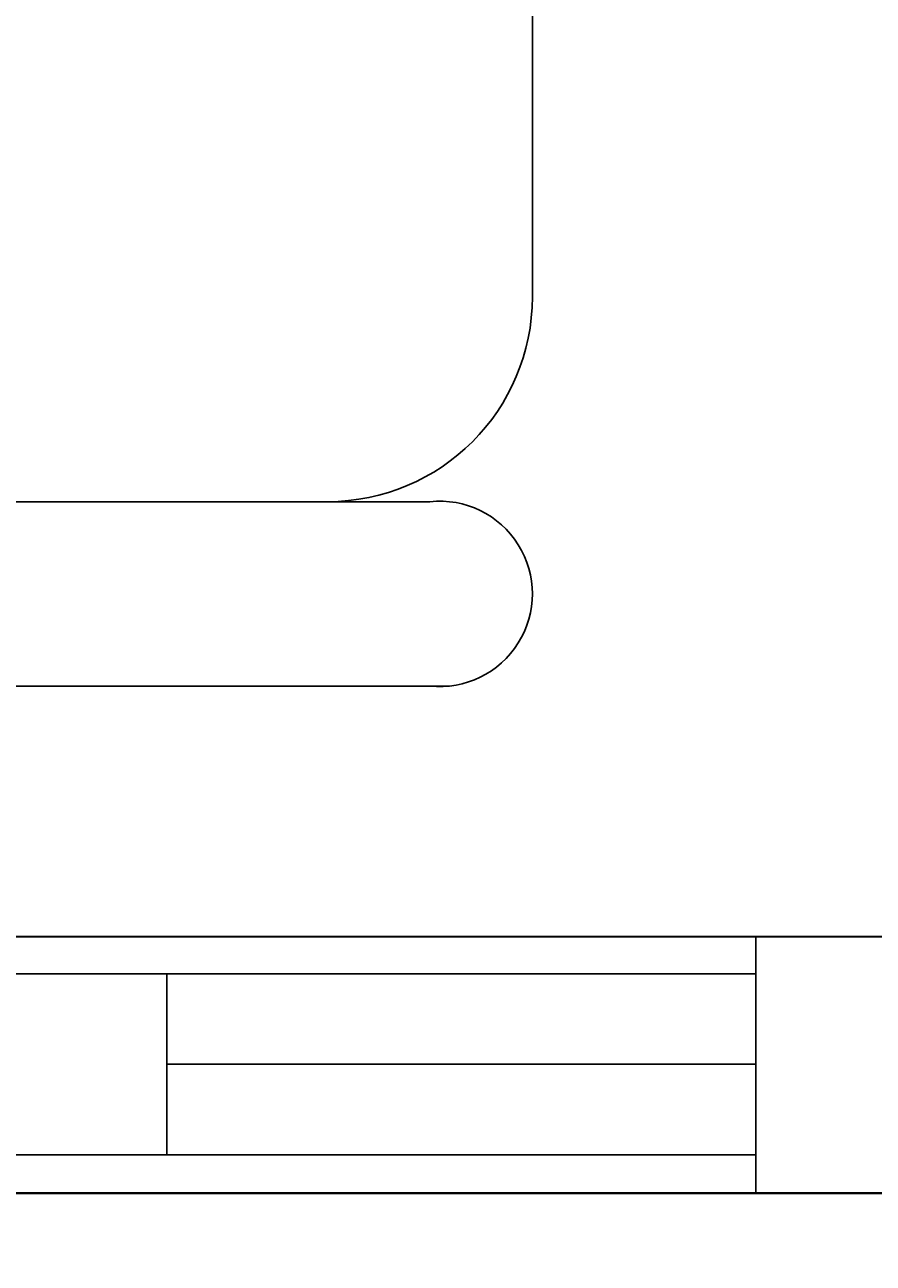
# Model space of a CAD drawing. Units: millimetres. Extents: x 19292 to 100733, y 12374 to 26974.
# Tile 4 of 24: x 28279 to 29028, y 14845 to 15938. Entities that reach past the tile are written whole.
import ezdxf

# ---------------------------------------------------------------- set-up
doc = ezdxf.new("R2010")
doc.units = ezdxf.units.MM
for name, color, linetype, lineweight in [('A-ANNO-DIMS', 2, 'Continuous', 18), ('A-FLOR-PATT', 252, 'Continuous', 13), ('A-FURN', 8, 'Continuous', 18), ('A-GLAZ', 3, 'Continuous', 25), ('A-WALL', 7, 'Continuous', 35)]:
    doc.layers.add(name, color=color, linetype=linetype, lineweight=lineweight)
doc.layers.add('FURNITURE', color=40, linetype='Continuous')
doc.layers.add('WINDOWS', color=50, linetype='Continuous')
doc.styles.get("Standard").update_dxf_attribs({"font": 'arial.ttf'})
doc.dimstyles.get("Standard").update_dxf_attribs({"dimtxt": 0.18, "dimasz": 0.18, "dimexe": 0.18, "dimexo": 0.0625, "dimgap": 0.09, "dimtad": 0, "dimtih": 1, "dimtoh": 1, "dimdec": 4, "dimzin": 0, "dimdsep": 46, "dimtxsty": 'Standard', "dimcen": 0.09, "dimadec": 0, "dimazin": 0, "dimtfac": 1, "dimtdec": 4, "dimtofl": 0, "dimtmove": 0, "dimatfit": 3, "dimfxl": 1, "dimtolj": 1, "dimtzin": 0, "dimarcsym": 0})

# ---------------------------------------------------------------- blocks, each defined once
blk = doc.blocks.new('WW')
at = {"layer": 'WINDOWS'}
for p, q in [((-5183.9, -4940.9), (-3983.9, -4940.9)), ((-4663.9, -4940.9), (-4663.9, -5100.9)), ((-4503.9, -4940.9), (-4503.9, -5100.9)), ((-4503.9, -4940.9), (-4503.9, -5100.9)), ((-5183.9, -5020.9), (-4663.9, -5020.9)), ((-4503.9, -5020.9), (-3983.9, -5020.9)), ((-5183.9, -5100.9), (-3983.9, -5100.9))]:
    blk.add_line(p, q, dxfattribs=at)
for points in [[(-5183.9, -5133.4), (-5183.9, -4908.4)], [(-3983.9, -4908.4), (-3983.9, -5133.4)]]:
    blk.add_lwpolyline(points, dxfattribs=at)
blk = doc.blocks.new('2sofa-hf')
at = {"layer": 'FURNITURE'}
for p, q in [((0, -23.849), (0, -12.325)), ((-16.2, -29.849), (-3, -29.849)), ((-21.6, -35.249), (-2.43, -35.249))]:
    blk.add_line(p, q, dxfattribs=at)
for centre, radius, start, end in [((-6, -23.849), 6, 270, 0), ((-2.715, -32.549), 2.715, 263.9744, 96.0256)]:
    blk.add_arc(centre, radius, start, end, dxfattribs=at)
blk = doc.blocks.new('*D79')
at = {"layer": 'A-ANNO-DIMS', "color": 0, "lineweight": -2, "transparency": 16777216}
for p, q in [((22694.1, 22860.7), (22694.1, 12808.8)), ((36144.2, 15985.7), (36144.2, 12808.8)), ((22694.3, 12809), (29418.7, 12809)), ((36144, 12809), (29419.6, 12809))]:
    blk.add_line(p, q, dxfattribs=at)
at = {"layer": 'A-ANNO-DIMS', "color": 0, "transparency": 16777216}
for points in [[(22694.3, 12809), (22694.3, 12809), (22694.1, 12809)], [(36144, 12809), (36144, 12809), (36144.2, 12809)]]:
    blk.add_solid(points, dxfattribs=at)
at = {"layer": 'Defpoints', "color": 0, "transparency": 16777216}
for p in [(22694.1, 22860.7), (36144.2, 15985.7), (36144.2, 12809)]:
    blk.add_point(p, dxfattribs=at)
at = {"layer": 'A-ANNO-DIMS', "color": 0, "transparency": 16777216, "insert": (29419.2, 12809), "char_height": 0.18, "attachment_point": 5}
blk.add_mtext('\\A1;13450', dxfattribs=at)
blk = doc.blocks.new('*D82')
at = {"layer": 'A-ANNO-DIMS', "color": 0, "lineweight": -2, "transparency": 16777216}
for p, q in [((27198.8, 13562.8), (27198.8, 23555.9)), ((27199, 23555.7), (29296.4, 23555.7)), ((31394.6, 23555.7), (29297.2, 23555.7)), ((31394.8, 13544.1), (31394.8, 23555.9))]:
    blk.add_line(p, q, dxfattribs=at)
at = {"layer": 'A-ANNO-DIMS', "color": 0, "transparency": 16777216}
for points in [[(27199, 23555.8), (27199, 23555.7), (27198.8, 23555.7)], [(31394.6, 23555.8), (31394.6, 23555.7), (31394.8, 23555.7)]]:
    blk.add_solid(points, dxfattribs=at)
at = {"layer": 'Defpoints', "color": 0, "transparency": 16777216}
for p in [(31394.8, 23555.7), (27198.8, 13562.7), (31394.8, 13544)]:
    blk.add_point(p, dxfattribs=at)
at = {"layer": 'A-ANNO-DIMS', "color": 0, "transparency": 16777216, "insert": (29296.8, 23555.7), "char_height": 0.18, "attachment_point": 5}
blk.add_mtext('\\A1;4196', dxfattribs=at)
blk = doc.blocks.new('*D86')
at = {"layer": 'A-ANNO-DIMS', "color": 0, "lineweight": -2, "transparency": 16777216}
for p, q in [((27198.8, 15132.8), (27198.8, 23555.9)), ((27199, 23555.7), (29198.5, 23555.7)), ((31198.6, 23555.7), (29199.2, 23555.7)), ((31198.8, 15132.8), (31198.8, 23555.9))]:
    blk.add_line(p, q, dxfattribs=at)
at = {"layer": 'A-ANNO-DIMS', "color": 0, "transparency": 16777216}
for points in [[(27199, 23555.8), (27199, 23555.7), (27198.8, 23555.7)], [(31198.6, 23555.8), (31198.6, 23555.7), (31198.8, 23555.7)]]:
    blk.add_solid(points, dxfattribs=at)
at = {"layer": 'Defpoints', "color": 0, "transparency": 16777216}
for p in [(31198.8, 23555.7), (27198.8, 15132.7), (31198.8, 15132.7)]:
    blk.add_point(p, dxfattribs=at)
at = {"layer": 'A-ANNO-DIMS', "color": 0, "transparency": 16777216, "insert": (29198.8, 23555.7), "char_height": 0.18, "attachment_point": 5}
blk.add_mtext('\\A1;4000', dxfattribs=at)

msp = doc.modelspace()

# ---------------------------------------------------------------- hatches: boundary and pattern name
at = {"layer": 'A-FLOR-PATT'}
h = msp.add_hatch(dxfattribs=at)
h.set_pattern_fill('CROSS', color=256, scale=40)
h.paths.add_polyline_path([(31394.799, 14906.403), (31051.542, 14906.403), (29468.571, 14906.403), (27198.815, 14906.403), (27198.815, 13543.993), (31394.799, 13543.993)])
h.paths.add_polyline_path([(27828.096, 14036.581), (30629.164, 14036.581), (30629.164, 14443.478), (27828.096, 14443.478)], flags=24)

# ---------------------------------------------------------------- linework, layer by layer
at = {"layer": 'A-WALL'}
for points in [[(29548.571, 14906.403), (27198.815, 14906.403), (27198.815, 13562.748), (23348.815, 13562.748), (23348.815, 19010.725), (22694.132, 19010.725), (22694.132, 22860.725), (28369.132, 22860.725), (28369.132, 21460.725), (31169.132, 21460.725), (31169.132, 22460.725), (34419.132, 22460.725), (34419.132, 22208.026)], [(29468.571, 15132.748), (27198.815, 15132.748), (27198.815, 17812.748)], [(31051.542, 14906.403), (31394.799, 14906.403), (31394.799, 13543.993), (27198.815, 13543.993), (27198.815, 14906.403), (29548.571, 14906.403)]]:
    msp.add_lwpolyline(points, dxfattribs=at)

# ---------------------------------------------------------------- block references
at = {"layer": 'A-FURN', "xscale": 30.13269765108242, "yscale": 30.13269765108242, "zscale": 30.13269765108242}
msp.add_blockref('2sofa-hf', (28726.739, 16416.302), dxfattribs=at)
at = {"layer": 'A-GLAZ'}
msp.add_blockref('WW', (32907.943, 20041.124), dxfattribs=at)

# ---------------------------------------------------------------- dimensions: what is measured, and where the dimension line sits
at = {"layer": 'A-ANNO-DIMS'}
for base, p1, p2, picture, middle in [((31394.799, 23555.725), (27198.815, 13562.748), (31394.799, 13543.993), '*D82', (29296.807, 23555.725)), ((31198.815, 23555.725), (27198.815, 15132.748), (31198.815, 15132.748), '*D86', (29198.815, 23555.725)), ((36144.169, 12808.993), (22694.132, 22860.725), (36144.169, 15985.725), '*D79', (29419.151, 12808.993))]:
    dim = msp.add_linear_dim(base=base, p1=p1, p2=p2, dimstyle='Standard', override={"dimdec": 0, "dimlfac": 1, "dimrnd": 0, "dimzin": 0, "dimdsep": 46, "dimlunit": 2}, dxfattribs=at)
    dim.commit()
    dim.dimension.update_dxf_attribs({"geometry": picture, "text_midpoint": middle})

doc.saveas('drawing.dxf')
